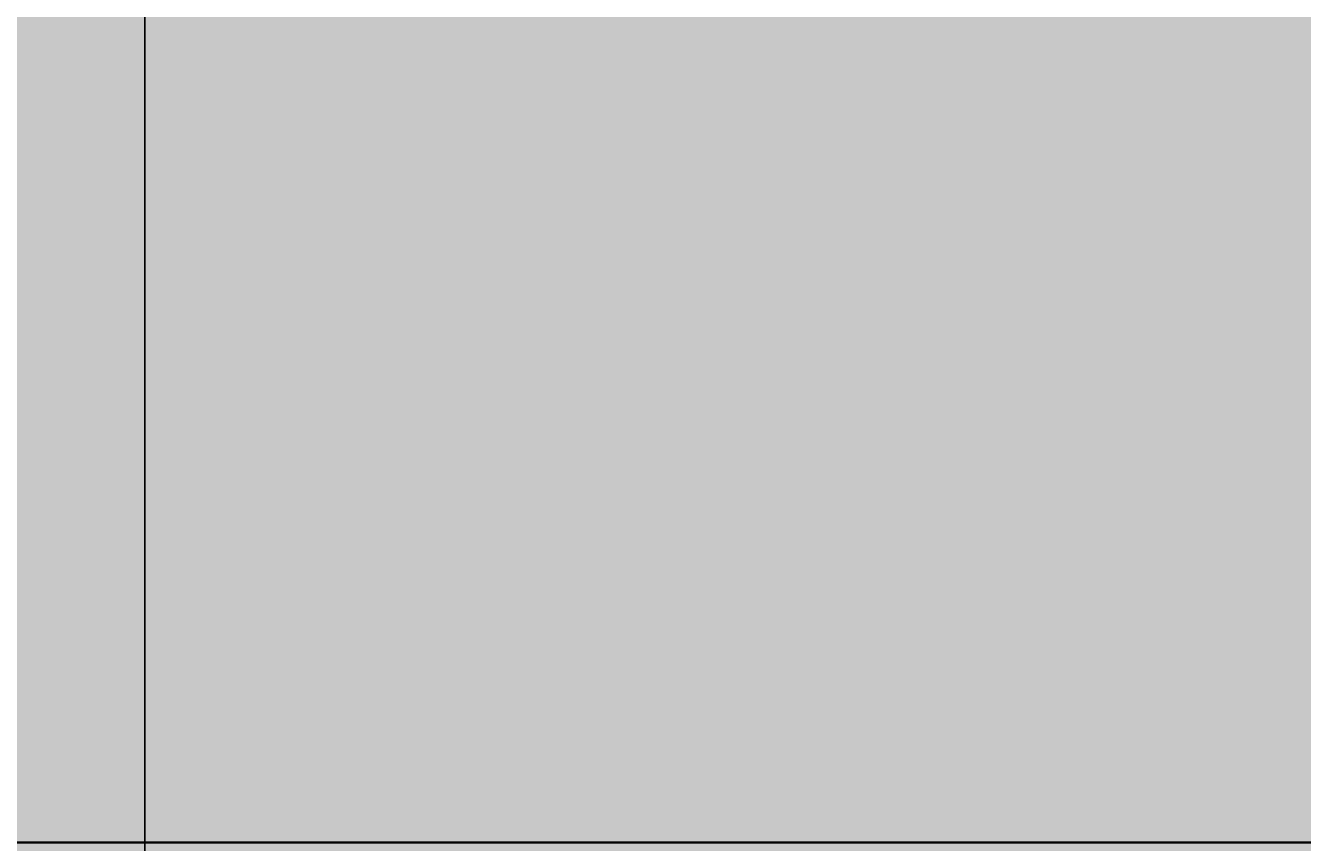
# Model space of a CAD drawing. Units: feet. Extents: x 2695 to 2912, y 795 to 1139.
# Tile 79 of 83: x 2840 to 2876, y 1063 to 1086. Entities that reach past the tile are written whole.
import ezdxf

# ---------------------------------------------------------------- set-up
doc = ezdxf.new("R2010")
doc.units = ezdxf.units.FT
for name, color, linetype, lineweight in [('A-ANNO-DIMS', 2, 'Continuous', 18), ('A-ELEV', 7, 'Continuous', 35), ('A-ELEV-PATT', 252, 'Continuous', 13)]:
    doc.layers.add(name, color=color, linetype=linetype, lineweight=lineweight)
doc.styles.get("Standard").update_dxf_attribs({"font": 'arial.ttf'})
doc.dimstyles.get("Standard").update_dxf_attribs({"dimtxt": 0.18, "dimasz": 0.18, "dimexe": 0.18, "dimexo": 0.0625, "dimgap": 0.09, "dimtad": 0, "dimtih": 1, "dimtoh": 1, "dimdec": 1, "dimzin": 0, "dimdsep": 46, "dimlunit": 3, "dimtxsty": 'Standard', "dimcen": 0.09, "dimadec": 0, "dimazin": 0, "dimtfac": 1, "dimtdec": 1, "dimtofl": 0, "dimtmove": 0, "dimatfit": 3, "dimfxl": 1, "dimtolj": 1, "dimtzin": 0, "dimarcsym": 0})

# ---------------------------------------------------------------- blocks, each defined once
blk = doc.blocks.new('*D10')
at = {"layer": 'A-ANNO-DIMS', "color": 0, "lineweight": -2, "transparency": 16777216}
for p, q in [((2778.034, 1020.886), (2778.034, 1138.886)), ((2778.214, 1138.706), (2810.411, 1138.706)), ((2843.395, 1138.706), (2811.198, 1138.706)), ((2843.575, 1020.886), (2843.575, 1138.886))]:
    blk.add_line(p, q, dxfattribs=at)
at = {"layer": 'A-ANNO-DIMS', "color": 0, "transparency": 16777216}
for points in [[(2778.214, 1138.736), (2778.214, 1138.676), (2778.034, 1138.706)], [(2843.395, 1138.736), (2843.395, 1138.676), (2843.575, 1138.706)]]:
    blk.add_solid(points, dxfattribs=at)
at = {"layer": 'Defpoints', "color": 0, "transparency": 16777216}
for p in [(2843.575, 1138.706), (2778.034, 1020.824), (2843.575, 1020.824)]:
    blk.add_point(p, dxfattribs=at)
at = {"layer": 'A-ANNO-DIMS', "color": 0, "transparency": 16777216, "insert": (2810.805, 1138.706), "char_height": 0.18, "attachment_point": 5}
blk.add_mtext('\\A1;65.54', dxfattribs=at)
blk = doc.blocks.new('*D11')
at = {"layer": 'A-ANNO-DIMS', "color": 0, "lineweight": -2, "transparency": 16777216}
for p, q in [((2843.575, 1020.886), (2843.575, 1138.886)), ((2843.755, 1138.706), (2869.128, 1138.706)), ((2895.289, 1138.706), (2869.916, 1138.706)), ((2895.469, 1107.898), (2895.469, 1138.886))]:
    blk.add_line(p, q, dxfattribs=at)
at = {"layer": 'A-ANNO-DIMS', "color": 0, "transparency": 16777216}
for points in [[(2843.755, 1138.736), (2843.755, 1138.676), (2843.575, 1138.706)], [(2895.289, 1138.736), (2895.289, 1138.676), (2895.469, 1138.706)]]:
    blk.add_solid(points, dxfattribs=at)
at = {"layer": 'Defpoints', "color": 0, "transparency": 16777216}
for p in [(2895.469, 1138.706), (2895.469, 1107.835), (2843.575, 1020.824)]:
    blk.add_point(p, dxfattribs=at)
at = {"layer": 'A-ANNO-DIMS', "color": 0, "transparency": 16777216, "insert": (2869.522, 1138.706), "char_height": 0.18, "attachment_point": 5}
blk.add_mtext('\\A1;51.89', dxfattribs=at)
blk = doc.blocks.new('*D50')
at = {"layer": 'A-ANNO-DIMS', "color": 0, "lineweight": -2, "transparency": 16777216}
for p, q in [((2810.041, 972.03), (2810.041, 1138.886)), ((2810.221, 1138.706), (2848.721, 1138.706)), ((2888.008, 1138.706), (2849.508, 1138.706)), ((2888.188, 972.03), (2888.188, 1138.886))]:
    blk.add_line(p, q, dxfattribs=at)
at = {"layer": 'A-ANNO-DIMS', "color": 0, "transparency": 16777216}
for points in [[(2810.221, 1138.736), (2810.221, 1138.676), (2810.041, 1138.706)], [(2888.008, 1138.736), (2888.008, 1138.676), (2888.188, 1138.706)]]:
    blk.add_solid(points, dxfattribs=at)
at = {"layer": 'Defpoints', "color": 0, "transparency": 16777216}
for p in [(2888.188, 1138.706), (2810.041, 971.967), (2888.188, 971.967)]:
    blk.add_point(p, dxfattribs=at)
at = {"layer": 'A-ANNO-DIMS', "color": 0, "transparency": 16777216, "insert": (2849.114, 1138.706), "char_height": 0.18, "attachment_point": 5}
blk.add_mtext('\\A1;78.15', dxfattribs=at)

msp = doc.modelspace()

# ---------------------------------------------------------------- hatches: boundary and pattern name
at = {"layer": 'A-ELEV-PATT'}
h = msp.add_hatch(color=256, dxfattribs=at)
h.set_gradient(color1=(255, 255, 255), tint=1)
h.paths.add_polyline_path([(2770.6361, 1122.9306), (2710.6361, 1122.9306), (2710.6361, 1118.4096), (2770.6361, 1118.4096)])
h.paths.add_polyline_path([(2890.6361, 1107.8588), (2770.6361, 1107.8588), (2770.6361, 1103.3378), (2890.6361, 1103.3378)])
h.paths.add_polyline_path([(2890.6361, 1062.9306), (2710.6361, 1062.9306), (2710.6361, 1056.9306), (2710.6361, 936.9306), (2710.6361, 924.3105), (2716.5358, 924.3105), (2890.6361, 924.3105), (2890.6361, 936.9306), (2715.8852, 936.9306), (2715.8852, 1050.3105), (2890.6361, 1050.3105)])
h.paths.add_polyline_path([(2716.5358, 924.3105), (2710.6361, 924.3105), (2710.6361, 810.9306), (2716.5358, 810.9306)])
h = msp.add_hatch(color=256, dxfattribs=at)
h.set_gradient(color1=(147, 149, 152), color2=(147, 149, 152), tint=1)
h.paths.add_polyline_path([(2770.6361, 1118.4096), (2710.6361, 1118.4096), (2710.6361, 1062.9306), (2770.6361, 1062.9306)])
h.paths.add_polyline_path([(2890.6361, 1103.3378), (2770.6361, 1103.3378), (2770.6361, 1062.9306), (2890.6361, 1062.9306)])
h.paths.add_polyline_path([(2730.7081, 1048.1052), (2755.1125, 1048.1052), (2755.1125, 936.9306), (2770.6361, 936.9306), (2770.6361, 1050.3105), (2715.8852, 1050.3105), (2715.8852, 936.9306), (2730.7081, 936.9306)])
h.paths.add_polyline_path([(2890.6361, 1050.3105), (2770.6361, 1050.3105), (2770.6361, 971.9673), (2778.0341, 971.9673), (2778.0341, 1020.8235), (2843.575, 1020.8235), (2843.575, 971.9673), (2890.6361, 971.9673)])
h.paths.add_polyline_path([(2888.1882, 970.7156), (2843.575, 970.7156), (2843.575, 964.8267), (2888.1882, 964.8267)])
h.paths.add_polyline_path([(2888.1882, 964.1328), (2843.575, 964.1328), (2843.575, 956.614), (2888.1882, 956.614)])
h.paths.add_polyline_path([(2888.1882, 955.9202), (2843.575, 955.9202), (2843.575, 949.2892), (2888.1882, 949.2892)])
h.paths.add_polyline_path([(2888.1882, 948.5954), (2843.575, 948.5954), (2843.575, 941.3507), (2888.1882, 941.3507)])
h.paths.add_polyline_path([(2888.1882, 940.6569), (2843.575, 940.6569), (2843.575, 936.9306), (2888.1882, 936.9306)])
h.paths.add_polyline_path([(2890.6361, 970.7156), (2888.9368, 970.7156), (2888.9368, 964.8267), (2890.6361, 964.8267)])
h.paths.add_polyline_path([(2890.6361, 964.1328), (2888.9368, 964.1328), (2888.9368, 956.614), (2890.6361, 956.614)])
h.paths.add_polyline_path([(2890.6361, 955.9202), (2888.9368, 955.9202), (2888.9368, 949.2892), (2890.6361, 949.2892)])
h.paths.add_polyline_path([(2890.6361, 940.6569), (2888.9368, 940.6569), (2888.9368, 936.9306), (2890.6361, 936.9306)])
h.paths.add_polyline_path([(2890.6361, 948.5954), (2888.9368, 948.5954), (2888.9368, 941.3507), (2890.6361, 941.3507)])
h.paths.add_polyline_path([(2772.5216, 970.7156), (2770.6361, 970.7156), (2770.6361, 964.8267), (2772.5216, 964.8267)])
h.paths.add_polyline_path([(2772.5216, 964.1328), (2770.6361, 964.1328), (2770.6361, 956.614), (2772.5216, 956.614)])
h.paths.add_polyline_path([(2772.5216, 955.9202), (2770.6361, 955.9202), (2770.6361, 949.2892), (2772.5216, 949.2892)])
h.paths.add_polyline_path([(2772.5216, 948.5954), (2770.6361, 948.5954), (2770.6361, 941.3507), (2772.5216, 941.3507)])
h.paths.add_polyline_path([(2772.5216, 940.6569), (2770.6361, 940.6569), (2770.6361, 936.9306), (2772.5216, 936.9306)])
h.paths.add_polyline_path([(2778.0341, 940.6569), (2773.2702, 940.6569), (2773.2702, 936.9306), (2778.0341, 936.9306)])
h.paths.add_polyline_path([(2778.0341, 970.7156), (2773.2702, 970.7156), (2773.2702, 964.8267), (2778.0341, 964.8267)])
h.paths.add_polyline_path([(2778.0341, 964.1328), (2773.2702, 964.1328), (2773.2702, 956.614), (2778.0341, 956.614)])
h.paths.add_polyline_path([(2778.0341, 955.9202), (2773.2702, 955.9202), (2773.2702, 949.2892), (2778.0341, 949.2892)])
h.paths.add_polyline_path([(2778.0341, 948.5954), (2773.2702, 948.5954), (2773.2702, 941.3507), (2778.0341, 941.3507)])
h.paths.add_polyline_path([(2810.0407, 940.6569), (2780.0341, 940.6569), (2780.0341, 936.9306), (2810.0407, 936.9306)])
h.paths.add_polyline_path([(2890.6361, 924.3105), (2770.6361, 924.3105), (2770.6361, 810.9306), (2773.5029, 810.9306), (2773.5029, 905.5143), (2805.9398, 905.5143), (2838.3767, 905.5143), (2838.3767, 810.9306), (2890.6361, 810.9306)])
h = msp.add_hatch(color=256, dxfattribs=at)
h.set_gradient(color1=(199, 200, 202), color2=(213, 227, 240), centered=1)
h.paths.add_polyline_path([(2890.6361, 1103.3378), (2770.6361, 1103.3378), (2770.6361, 1062.9306), (2890.6361, 1062.9306)])

# ---------------------------------------------------------------- linework, layer by layer
at = {"layer": 'A-ELEV'}
for q in [(2890.6361, 1062.9306), (2895.4694, 1062.9306)]:
    msp.add_line((2710.6361, 1062.9306), q, dxfattribs=at)

# ---------------------------------------------------------------- dimensions: what is measured, and where the dimension line sits
at = {"layer": 'A-ANNO-DIMS'}
for base, p1, p2, picture, middle in [((2843.575, 1138.7056), (2778.0341, 1020.8235), (2843.575, 1020.8235), '*D10', (2810.8045, 1138.7056)), ((2888.1882, 1138.7056), (2810.0407, 971.9673), (2888.1882, 971.9673), '*D50', (2849.1144, 1138.7056)), ((2895.4694, 1138.7056), (2843.575, 1020.8235), (2895.4694, 1107.8352), '*D11', (2869.5222, 1138.7056))]:
    dim = msp.add_linear_dim(base=base, p1=p1, p2=p2, dimstyle='Standard', override={"dimdec": 2, "dimlfac": 1, "dimrnd": 0, "dimzin": 0, "dimdsep": 46, "dimlunit": 2}, dxfattribs=at)
    dim.commit()
    dim.dimension.update_dxf_attribs({"geometry": picture, "text_midpoint": middle})

doc.saveas('drawing.dxf')
